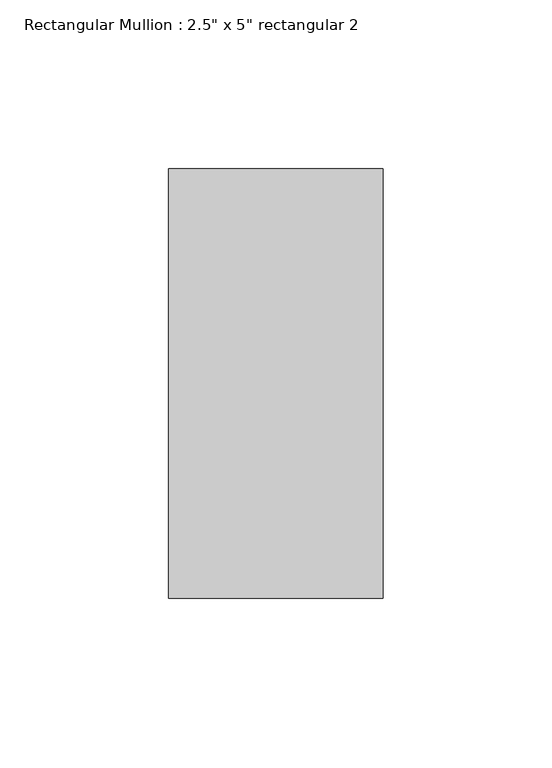
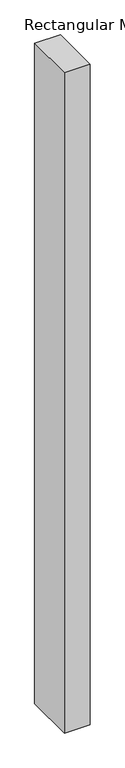
"""IFC4 building model written with IfcOpenShell, lengths in millimetres: member geometry."""

from ifc_helpers import new_model, si_unit, frame, origin, place, context, project, spatial, polyline, outline, extrude, source, transform, mapped, element, save


def member_14ac651b(model_context):
    return source(origin(), model_context, "Body", "SweptSolid", [
        extrude(outline(polyline([(0.0, 63.5), (0.0, -63.5), (-63.5, -63.5), (-63.5, 63.5), (0.0, 63.5)])), frame((0.0, 0.0, -1720.9224616), z_axis=(0.0, 0.0, 1.0), x_axis=(1.0, 0.0, 0.0)), (0.0, 0.0, 1.0), 1720.9224616),
    ])


if __name__ == "__main__":
    model = new_model("IFC4")
    model_context = context("Model", 3, world=origin())
    ifc_project = project(units=[si_unit("LENGTHUNIT", "METRE", prefix="MILLI")], contexts=[model_context])
    site = spatial("IfcSite", under=ifc_project)
    building = spatial("IfcBuilding", under=site)
    placement = place(None, origin())
    member_shape = member_14ac651b(model_context)
    element("IfcMember", 1, ObjectType="Rectangular Mullion : 2.5\" x 5\" rectangular 2", at=placement, inside=building, context=model_context, shape_type="MappedRepresentation", body=[
        mapped(member_shape, transform((0.0, 0.0, 0.0), x_axis=(1.0, 0.0, 0.0), y_axis=(0.0, 1.0, 0.0), z_axis=(0.0, 0.0, 1.0))),
    ])
    save(model, "model.ifc")

# Revit data of these elements
# Type "Rectangular Mullion : 2.5\" x 5\" rectangular 2"
#   built-in parameter 1007304 = 0.416667 (stored number, unit not read)
#   built-in parameter 1007301 = 0.104167 (stored number, unit not read)
#   built-in parameter 1007300 = 0.104167 (stored number, unit not read)
